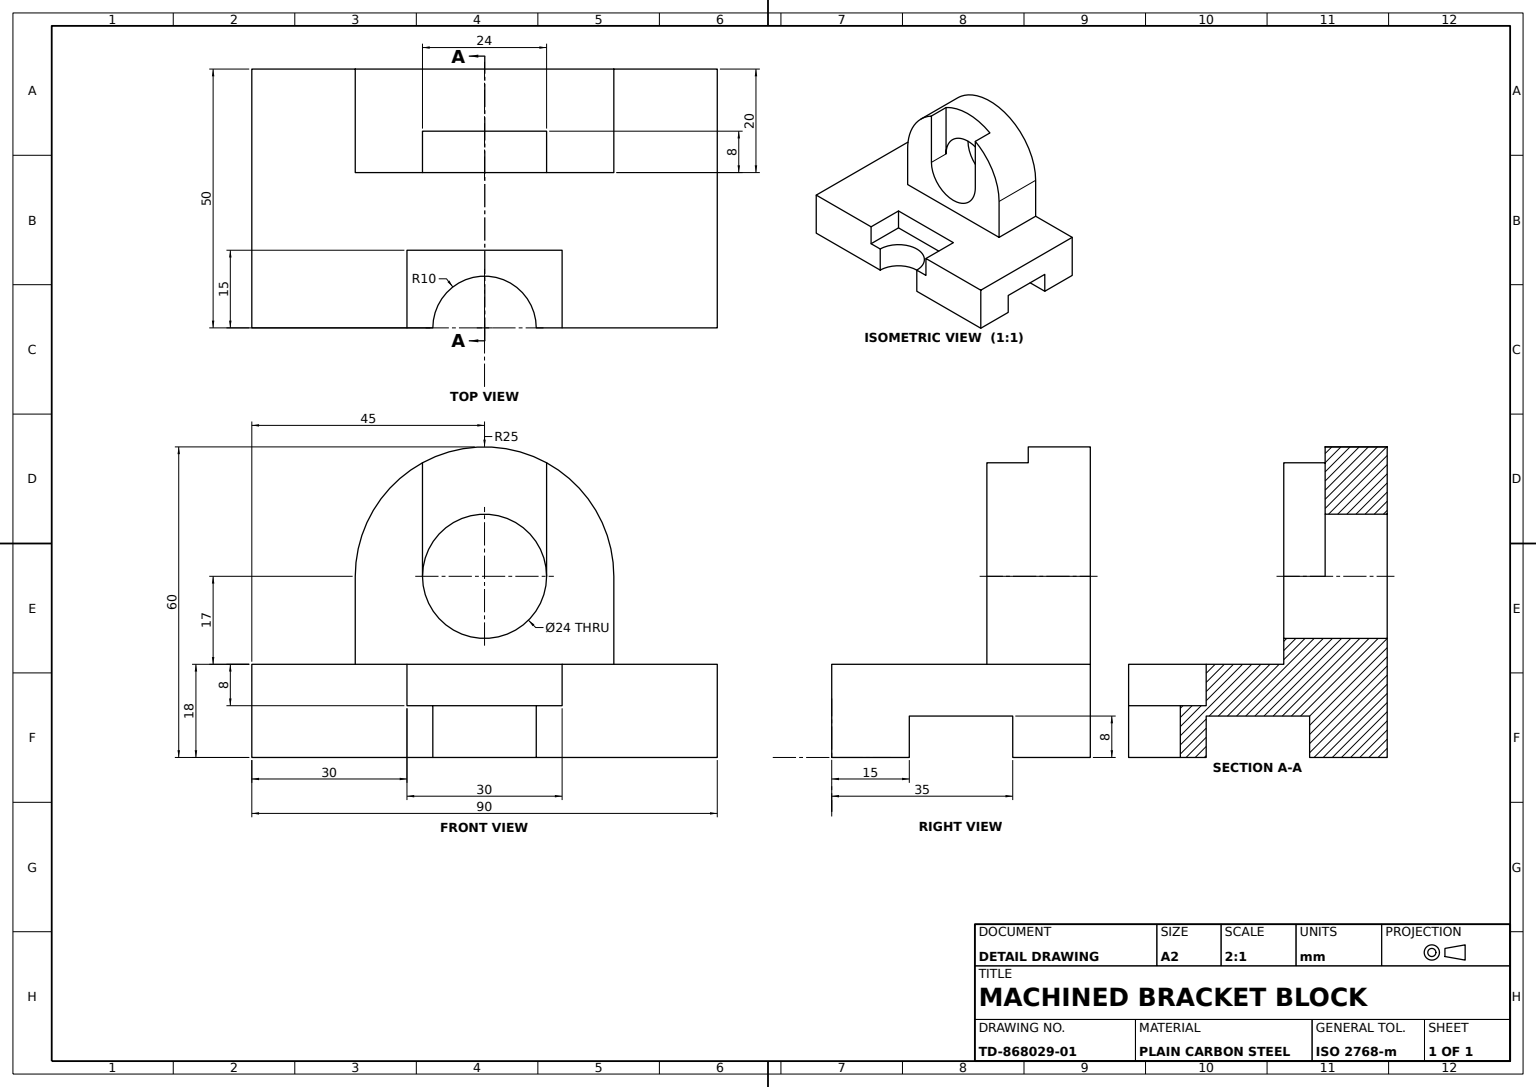
from build123d import *

# Parameters (mm, degrees)
BASE_PLATE_SKETCH_W       = 90
BASE_PLATE_SKETCH_H       = 18
BASE_PLATE_90X18X50_DEPTH = 50
PIVOT_LUG_SKETCH_R        = 12
PIVOT_LUG_DEPTH           = 20
BOTTOM_GROOVE_SKETCH_W    = 20
BOTTOM_GROOVE_SKETCH_H    = 8
BOTTOM_GROOVE_DEPTH       = 120.163752878
LUG_START                 = -8
LUG_SLOT_DEPTH            = 8
TOP_POCKET_SKETCH_W       = 30
TOP_POCKET_SKETCH_H       = 15
TOP_POCKET_DEPTH          = 8
POCKET_HOLE_20_SKETCH_R   = 10
POCKET_HOLE_20_DEPTH      = 115.455231423


with BuildPart() as part:
    # Base Plate Sketch → Base Plate 90x18x50 (new body)
    with BuildSketch(Plane.XY):
        with Locations((45, 9)):
            Rectangle(BASE_PLATE_SKETCH_W, BASE_PLATE_SKETCH_H)
    extrude(amount=BASE_PLATE_90X18X50_DEPTH)

    # Pivot Lug Sketch → Pivot Lug (add)
    with BuildSketch(Plane.XY):
        with BuildLine():
            Line((20, 35), (20, 18))
            Line((20, 18), (70, 18))
            Line((70, 18), (70, 35))
            ThreePointArc((70, 35), (45, 60), (20, 35))
        make_face()
        with Locations((45, 35)):
            Circle(PIVOT_LUG_SKETCH_R, mode=Mode.SUBTRACT)
    extrude(amount=PIVOT_LUG_DEPTH)

    # Bottom Groove Sketch → Bottom Groove (cut, through all)
    with BuildSketch(Plane(origin=(90, 0, 0), x_dir=(0, 0, -1), z_dir=(1, 0, 0))):
        with Locations((-25, 4)):
            Rectangle(BOTTOM_GROOVE_SKETCH_W, BOTTOM_GROOVE_SKETCH_H)
    extrude(amount=-BOTTOM_GROOVE_DEPTH, mode=Mode.SUBTRACT)

    # Lug Slot Sketch → Lug Slot (cut)
    with BuildSketch(Plane.XY.offset(20).offset(LUG_START)):
        with BuildLine():
            Line((33, 35), (33, 56.931712199))
            ThreePointArc((33, 56.931712199), (45, 60), (57, 56.931712199))
            Line((57, 56.931712199), (57, 35))
            ThreePointArc((57, 35), (45, 47), (33, 35))
        make_face()
    extrude(amount=LUG_SLOT_DEPTH, mode=Mode.SUBTRACT)

    # Top Pocket Sketch → Top Pocket (cut)
    with BuildSketch(Plane(origin=(0, 18, 0), x_dir=(1, 0, 0), z_dir=(0, 1, 0))):
        with Locations((45, -42.5)):
            Rectangle(TOP_POCKET_SKETCH_W, TOP_POCKET_SKETCH_H)
    extrude(amount=-TOP_POCKET_DEPTH, mode=Mode.SUBTRACT)

    # Pocket Hole Ø20 Sketch → Pocket Hole Ø20 (cut, through all)
    with BuildSketch(Plane(origin=(0, 10, 0), x_dir=(1, 0, 0), z_dir=(0, 1, 0))):
        with Locations((45, -50)):
            Circle(POCKET_HOLE_20_SKETCH_R)
    extrude(amount=-POCKET_HOLE_20_DEPTH, mode=Mode.SUBTRACT)


solid = part.part
